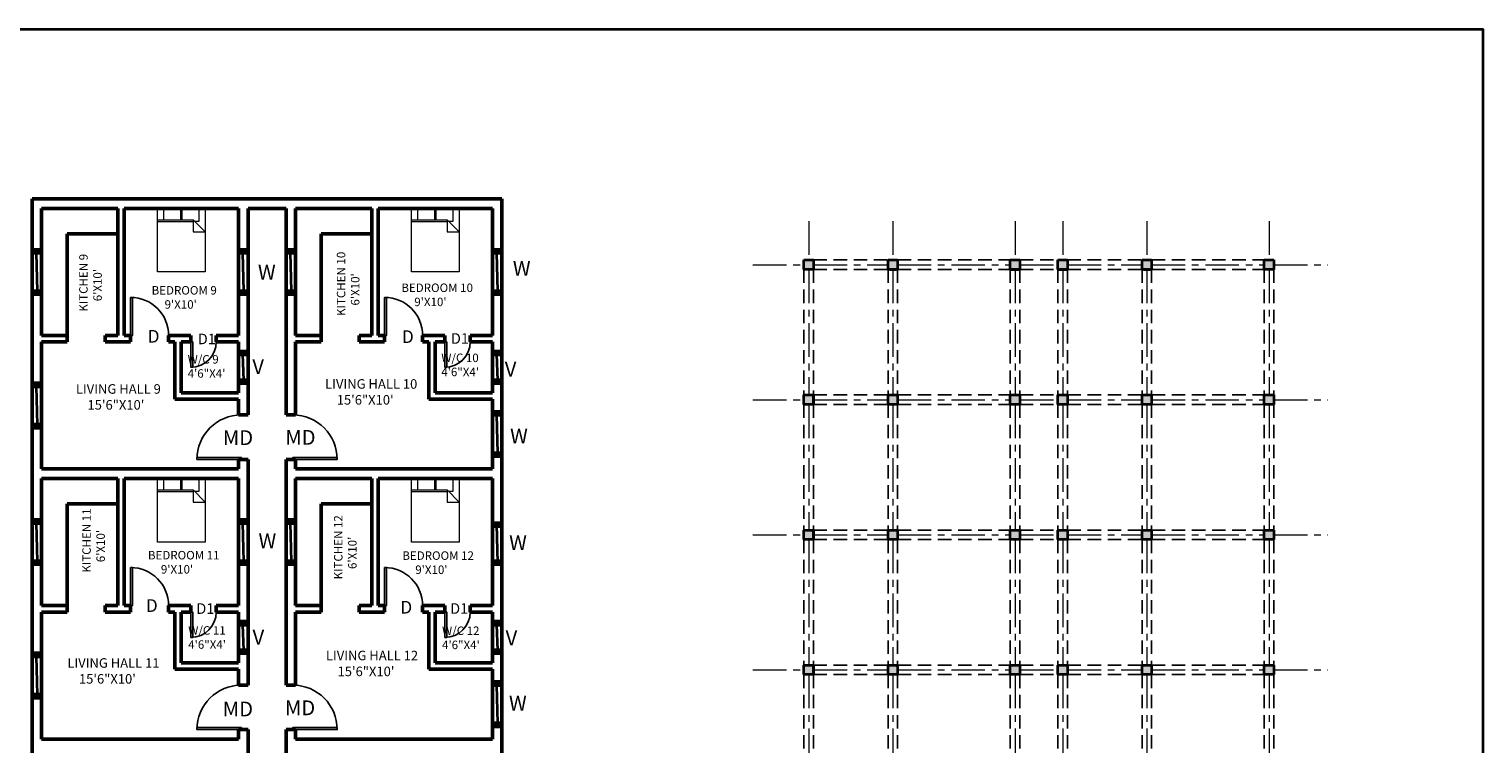
# Model space of a CAD drawing. Units: inches. Extents: x 9239 to 26065, y 6728 to 14611.
# Tile 12 of 12: x 24691 to 26065, y 13937 to 14611. Entities that reach past the tile are written whole.
import ezdxf

# ---------------------------------------------------------------- set-up
doc = ezdxf.new("R2010")
doc.units = ezdxf.units.IN
doc.header["$MEASUREMENT"] = 0
doc.linetypes.add('CENTER', pattern=[50.8, 31.75, -6.35, 6.35, -6.35])
doc.linetypes.add('DASHED', pattern=[19.05, 12.7, -6.35])
for name, color, linetype, lineweight in [('A-ANNO-TEXT', 7, 'Continuous', 18), ('A-ANNO-TTLB', 7, 'Continuous', 35), ('A-AREA-IDEN', 7, 'Continuous', 18), ('A-DOOR', 4, 'Continuous', 25), ('A-FURN', 8, 'Continuous', 18), ('A-GLAZ', 4, 'Continuous', 25), ('A-GRID', 3, 'CENTER', 18), ('A-WALL', 7, 'Continuous', 50), ('S-BEAM', 4, 'DASHED', 25), ('S-COLS', 1, 'Continuous', 35), ('S-PATT', 252, 'Continuous', 13)]:
    doc.layers.add(name, color=color, linetype=linetype, lineweight=lineweight)
doc.styles.get("Standard").update_dxf_attribs({"font": 'arial.ttf'})

# ---------------------------------------------------------------- blocks, each defined once
blk = doc.blocks.new('*U10')
for p, q in [((0, 0), (0, -6)), ((36, 0), (36, -6))]:
    blk.add_line(p, q)
blk.add_lwpolyline([(0, 0), (0, 36), (1.75, 36), (1.75, 0)], close=True)
blk.add_arc((0, 0), 36, 0, 90)
blk = doc.blocks.new('*U34')
for p, q in [((0, 0), (0, 6)), ((24, 0), (24, 6))]:
    blk.add_line(p, q)
blk.add_lwpolyline([(0, 0), (0, -24), (1.75, -24), (1.75, 0)], close=True)
blk.add_arc((0, 0), 24, 270, 0)
blk = doc.blocks.new('*U33')
for p, q in [((-40, 0), (-40, 6)), ((0, 0), (0, 6))]:
    blk.add_line(p, q)
blk.add_lwpolyline([(0, 0), (0, -40), (-1.75, -40), (-1.75, 0)], close=True)
blk.add_arc((0, 0), 40, 180, 270)
blk = doc.blocks.new('*U35')
for p, q in [((0, 0), (0, -6)), ((-40, 0), (-40, -6))]:
    blk.add_line(p, q)
blk.add_lwpolyline([(0, 0), (0, 40), (-1.75, 40), (-1.75, 0)], close=True)
blk.add_arc((0, 0), 40, 90, 180)
blk = doc.blocks.new('Bed - Queen')
for p, q in [((0, -80.00003), (0, 0)), ((0, 0), (59.99999, 0)), ((59.99999, 0), (59.99999, -80.00003)), ((0, -14.4), (44.8, -14.4)), ((44.8, -16.8), (0, -16.8)), ((7.99999, -1.2), (28.79998, -1.2)), ((7.99999, -14.4), (7.99999, -1.2)), ((28.79998, -1.2), (28.79998, -14.4)), ((31.19999, -1.2), (51.99999, -1.2)), ((31.19999, -14.4), (31.19999, -1.2)), ((59.99999, -29.6), (44.8, -14.4)), ((44.8, -14.4), (44.8, -29.6)), ((51.99999, -16.4), (46.79936, -16.4)), ((51.99999, -1.2), (51.99999, -16.4)), ((44.8, -29.6), (59.99999, -29.6)), ((59.99999, -80.00003), (0, -80.00003))]:
    blk.add_line(p, q)
blk = doc.blocks.new('WIN-36')
for p, q in [((0, 1), (36, 1)), ((0, 0.5), (36, 0.5)), ((0, 0), (36, 0))]:
    blk.add_line(p, q)
blk = doc.blocks.new('WIN-24')
for p, q in [((0, 1), (24, 1)), ((0, 0.5), (24, 0.5)), ((0, 0), (24, 0))]:
    blk.add_line(p, q)

msp = doc.modelspace()

# ---------------------------------------------------------------- hatches: boundary and pattern name
at = {"layer": 'S-PATT'}
h = msp.add_hatch(color=256, dxfattribs=at)
h.dxf.hatch_style = 1
h.paths.add_polyline_path([(25432.02, 14384.38), (25432.02, 14393.38), (25423.02, 14393.38), (25423.02, 14384.38)])
h.paths.add_polyline_path([(25511.52, 14384.38), (25511.52, 14393.38), (25502.52, 14393.38), (25502.52, 14384.38)])
h.paths.add_polyline_path([(25627.02, 14384.38), (25627.02, 14393.38), (25618.02, 14393.38), (25618.02, 14384.38)])
h.paths.add_polyline_path([(25672.02, 14393.38), (25663.02, 14393.38), (25663.02, 14384.38), (25672.02, 14384.38)])
h.paths.add_polyline_path([(25742.52, 14384.38), (25751.52, 14384.38), (25751.52, 14393.38), (25742.52, 14393.38)])
h.paths.add_polyline_path([(25858.02, 14384.38), (25867.02, 14384.38), (25867.02, 14393.38), (25858.02, 14393.38)])
h.paths.add_polyline_path([(25423.02, 14256.88), (25432.02, 14256.88), (25432.02, 14265.88), (25423.02, 14265.88)])
h.paths.add_polyline_path([(25502.52, 14256.88), (25511.52, 14256.88), (25511.52, 14265.88), (25502.52, 14265.88)])
h.paths.add_polyline_path([(25618.02, 14256.88), (25627.02, 14256.88), (25627.02, 14265.88), (25618.02, 14265.88)])
h.paths.add_polyline_path([(25672.02, 14265.88), (25663.02, 14265.88), (25663.02, 14256.88), (25672.02, 14256.88)])
h.paths.add_polyline_path([(25751.52, 14256.88), (25751.52, 14265.88), (25742.52, 14265.88), (25742.52, 14256.88)])
h.paths.add_polyline_path([(25858.02, 14256.88), (25867.02, 14256.88), (25867.02, 14265.88), (25858.02, 14265.88)])
h.paths.add_polyline_path([(25423.02, 14129.38), (25432.02, 14129.38), (25432.02, 14138.38), (25423.02, 14138.38)])
h.paths.add_polyline_path([(25511.52, 14129.38), (25511.52, 14138.38), (25502.52, 14138.38), (25502.52, 14129.38)])
h.paths.add_polyline_path([(25618.02, 14129.38), (25627.02, 14129.38), (25627.02, 14138.38), (25618.02, 14138.38)])
h.paths.add_polyline_path([(25672.02, 14138.38), (25663.02, 14138.38), (25663.02, 14129.38), (25672.02, 14129.38)])
h.paths.add_polyline_path([(25742.52, 14129.38), (25751.52, 14129.38), (25751.52, 14138.38), (25742.52, 14138.38)])
h.paths.add_polyline_path([(25867.02, 14129.38), (25867.02, 14138.38), (25858.02, 14138.38), (25858.02, 14129.38)])
h.paths.add_polyline_path([(25432.02, 14010.88), (25423.02, 14010.88), (25423.02, 14001.88), (25432.02, 14001.88)])
h.paths.add_polyline_path([(25502.52, 14010.88), (25502.52, 14001.88), (25511.52, 14001.88), (25511.52, 14010.88)])
h.paths.add_polyline_path([(25618.02, 14001.88), (25627.02, 14001.88), (25627.02, 14010.88), (25618.02, 14010.88)])
h.paths.add_polyline_path([(25672.02, 14001.88), (25672.02, 14010.88), (25663.02, 14010.88), (25663.02, 14001.88)])
h.paths.add_polyline_path([(25751.52, 14010.88), (25742.52, 14010.88), (25742.52, 14001.88), (25751.52, 14001.88)])
h.paths.add_polyline_path([(25867.02, 14010.88), (25858.02, 14010.88), (25858.02, 14001.88), (25867.02, 14001.88)])
h.paths.add_polyline_path([(25432.02, 13874.38), (25432.02, 13883.38), (25423.02, 13883.38), (25423.02, 13874.38)])
h.paths.add_polyline_path([(25502.52, 13874.38), (25511.52, 13874.38), (25511.52, 13883.38), (25502.52, 13883.38)])
h.paths.add_polyline_path([(25627.02, 13883.38), (25618.02, 13883.38), (25618.02, 13874.38), (25627.02, 13874.38)])
h.paths.add_polyline_path([(25672.02, 13874.38), (25672.02, 13883.38), (25663.02, 13883.38), (25663.02, 13874.38)])
h.paths.add_polyline_path([(25751.52, 13883.38), (25742.52, 13883.38), (25742.52, 13874.38), (25751.52, 13874.38)])
h.paths.add_polyline_path([(25858.02, 13874.38), (25867.02, 13874.38), (25867.02, 13883.38), (25858.02, 13883.38)])
h.paths.add_polyline_path([(25432.02, 13746.88), (25432.02, 13755.88), (25423.02, 13755.88), (25423.02, 13746.88)])
h.paths.add_polyline_path([(25502.52, 13747.4), (25511.52, 13747.4), (25511.52, 13756.4), (25502.52, 13756.4)])
h.paths.add_polyline_path([(25627.02, 13746.88), (25627.02, 13755.88), (25618.02, 13755.88), (25618.02, 13746.88)])
h.paths.add_polyline_path([(25672.02, 13746.88), (25672.02, 13755.88), (25663.02, 13755.88), (25663.02, 13746.88)])
h.paths.add_polyline_path([(25742.52, 13746.88), (25751.52, 13746.88), (25751.52, 13755.88), (25742.52, 13755.88)])
h.paths.add_polyline_path([(25867.02, 13746.88), (25867.02, 13755.88), (25858.02, 13755.88), (25858.02, 13746.88)])
h.paths.add_polyline_path([(25423.02, 13619.38), (25432.02, 13619.38), (25432.02, 13628.38), (25423.02, 13628.38)])
h.paths.add_polyline_path([(25511.52, 13619.38), (25511.52, 13628.38), (25502.52, 13628.38), (25502.52, 13619.38)])
h.paths.add_polyline_path([(25627.02, 13619.38), (25627.02, 13628.38), (25618.02, 13628.38), (25618.02, 13619.38)])
h.paths.add_polyline_path([(25672.02, 13619.38), (25672.02, 13628.38), (25663.02, 13628.38), (25663.02, 13619.38)])
h.paths.add_polyline_path([(25751.52, 13628.38), (25742.52, 13628.38), (25742.52, 13619.38), (25751.52, 13619.38)])
h.paths.add_polyline_path([(25858.02, 13619.38), (25867.02, 13619.38), (25867.02, 13628.38), (25858.02, 13628.38)])
h.paths.add_polyline_path([(25423.02, 13491.88), (25432.02, 13491.88), (25432.02, 13500.88), (25423.02, 13500.88)])
h.paths.add_polyline_path([(25511.52, 13500.88), (25502.52, 13500.88), (25502.52, 13491.88), (25511.52, 13491.88)])
h.paths.add_polyline_path([(25627.02, 13491.88), (25627.02, 13500.88), (25618.02, 13500.88), (25618.02, 13491.88)])
h.paths.add_polyline_path([(25663.02, 13491.88), (25672.02, 13491.88), (25672.02, 13500.88), (25663.02, 13500.88)])
h.paths.add_polyline_path([(25742.52, 13491.88), (25751.52, 13491.88), (25751.52, 13500.88), (25742.52, 13500.88)])
h.paths.add_polyline_path([(25432.02, 13373.38), (25423.02, 13373.38), (25423.02, 13364.38), (25432.02, 13364.38)])
h.paths.add_polyline_path([(25502.52, 13373.38), (25502.52, 13364.38), (25511.52, 13364.38), (25511.52, 13373.38)])
h.paths.add_polyline_path([(25618.02, 13373.38), (25618.02, 13364.38), (25627.02, 13364.38), (25627.02, 13373.38)])
h.paths.add_polyline_path([(25663.02, 13373.38), (25663.02, 13364.38), (25672.02, 13364.38), (25672.02, 13373.38)])
h.paths.add_polyline_path([(25742.52, 13373.38), (25742.52, 13364.38), (25751.52, 13364.38), (25751.52, 13373.38)])
h.paths.add_polyline_path([(25858.02, 13373.38), (25858.02, 13364.38), (25867.02, 13364.38), (25867.02, 13373.38)])
h.paths.add_polyline_path([(25432.02, 13298.38), (25423.02, 13298.38), (25423.02, 13289.38), (25432.02, 13289.38)])
h.paths.add_polyline_path([(25511.52, 13298.38), (25502.52, 13298.38), (25502.52, 13289.38), (25511.52, 13289.38)])
h.paths.add_polyline_path([(25618.02, 13298.38), (25618.02, 13289.38), (25627.02, 13289.38), (25627.02, 13298.38)])
h.paths.add_polyline_path([(25663.02, 13298.38), (25663.02, 13289.38), (25672.02, 13289.38), (25672.02, 13298.38)])
h.paths.add_polyline_path([(25742.52, 13298.38), (25742.52, 13289.38), (25751.52, 13289.38), (25751.52, 13298.38)])
h.paths.add_polyline_path([(25858.02, 13298.38), (25858.02, 13289.38), (25867.02, 13289.38), (25867.02, 13298.38)])

# ---------------------------------------------------------------- linework, layer by layer
at = {"layer": 'A-ANNO-TTLB'}
msp.add_lwpolyline([(23324.14, 14611.25), (26064.6, 14611.25), (26064.6, 11591.84), (23324.14, 11591.84)], close=True, dxfattribs=at)
at = {"layer": 'A-GRID'}
for p, q in [((25427.52, 14430.01), (25427.52, 14393.38)), ((25507.02, 14430.01), (25507.02, 14393.38)), ((25622.52, 14430.01), (25622.52, 14393.38)), ((25667.52, 14430.01), (25667.52, 14393.38)), ((25747.02, 14430.01), (25747.02, 14393.38)), ((25862.52, 14430.01), (25862.52, 14393.38)), ((25374.85, 14388.88), (25423.02, 14388.88)), ((25427.52, 14384.38), (25427.52, 14265.88)), ((25432.02, 14388.88), (25502.52, 14388.88)), ((25507.02, 14384.38), (25507.02, 14265.88)), ((25511.52, 14388.88), (25618.02, 14388.88)), ((25622.52, 14384.38), (25622.52, 14265.88)), ((25627.02, 14388.88), (25663.02, 14388.88)), ((25667.52, 14384.38), (25667.52, 14265.88)), ((25672.02, 14388.88), (25742.52, 14388.88)), ((25747.02, 14384.38), (25747.02, 14265.88)), ((25751.52, 14388.88), (25858.02, 14388.88)), ((25862.52, 14384.38), (25862.52, 14265.88)), ((25867.02, 14388.88), (25917.98, 14388.88)), ((25374.85, 14261.38), (25423.02, 14261.38)), ((25432.02, 14261.38), (25502.52, 14261.38)), ((25511.52, 14261.38), (25618.02, 14261.38)), ((25627.02, 14261.38), (25663.02, 14261.38)), ((25672.02, 14261.38), (25742.52, 14261.38)), ((25751.52, 14261.38), (25858.02, 14261.38)), ((25867.02, 14261.38), (25917.98, 14261.38)), ((25427.52, 14256.88), (25427.52, 14138.38)), ((25507.02, 14256.88), (25507.02, 14138.38)), ((25622.52, 14256.88), (25622.52, 14138.38)), ((25667.52, 14256.88), (25667.52, 14138.38)), ((25747.02, 14256.88), (25747.02, 14138.38)), ((25862.52, 14256.88), (25862.52, 14138.38)), ((25374.85, 14133.88), (25423.02, 14133.88)), ((25427.52, 14129.38), (25427.52, 14010.88)), ((25432.02, 14133.88), (25502.52, 14133.88)), ((25507.02, 14129.38), (25507.02, 14010.88)), ((25511.52, 14133.88), (25618.02, 14133.88)), ((25622.52, 14129.38), (25622.52, 14010.88)), ((25627.02, 14133.88), (25663.02, 14133.88)), ((25667.52, 14129.38), (25667.52, 14010.88)), ((25672.02, 14133.88), (25742.52, 14133.88)), ((25747.02, 14129.38), (25747.02, 14010.88)), ((25751.52, 14133.88), (25858.02, 14133.88)), ((25862.52, 14129.38), (25862.52, 14010.88)), ((25867.02, 14133.88), (25917.98, 14133.88)), ((25374.85, 14006.38), (25423.02, 14006.38)), ((25427.52, 14001.88), (25427.52, 13883.38)), ((25432.02, 14006.38), (25502.52, 14006.38)), ((25507.02, 14001.88), (25507.02, 13883.38)), ((25511.52, 14006.38), (25618.02, 14006.38)), ((25622.52, 14001.88), (25622.52, 13883.38)), ((25627.02, 14006.38), (25663.02, 14006.38)), ((25667.52, 14001.88), (25667.52, 13883.38)), ((25672.02, 14006.38), (25742.52, 14006.38)), ((25747.02, 14001.88), (25747.02, 13883.38)), ((25751.52, 14006.38), (25858.02, 14006.38)), ((25862.52, 14001.88), (25862.52, 13883.38)), ((25867.02, 14006.38), (25917.98, 14006.38))]:
    msp.add_line(p, q, dxfattribs=at)
at = {"layer": 'A-WALL'}
for p, q in [((24693.68, 14451.02), (25137.68, 14451.02)), ((24693.68, 13347.02), (24693.68, 14451.02)), ((24702.68, 14442.02), (24774.68, 14442.02)), ((24702.68, 14322.02), (24702.68, 14442.02)), ((24774.68, 14322.02), (24774.68, 14442.02)), ((24780.68, 14322.02), (24780.68, 14442.02)), ((24780.68, 14442.02), (24888.68, 14442.02)), ((24888.68, 14322.02), (24888.68, 14442.02)), ((24897.68, 14247.02), (24897.68, 14442.02)), ((24897.68, 14442.02), (24933.68, 14442.02)), ((24933.68, 14442.02), (24933.68, 14247.02)), ((24942.68, 14442.02), (24942.68, 14322.02)), ((24942.68, 14442.02), (25014.68, 14442.02)), ((25014.68, 14442.02), (25014.68, 14322.02)), ((25020.68, 14442.02), (25020.68, 14322.02)), ((25020.68, 14442.02), (25128.68, 14442.02)), ((25128.68, 14442.02), (25128.68, 14322.02)), ((25137.68, 14451.02), (25137.68, 13347.02)), ((24726.68, 14322.02), (24726.68, 14418.02)), ((24726.68, 14418.02), (24774.68, 14418.02)), ((24966.68, 14418.02), (24966.68, 14322.02)), ((24966.68, 14418.02), (25014.68, 14418.02)), ((24702.68, 14403.02), (24693.68, 14403.02)), ((24702.68, 14400.02), (24693.68, 14400.02)), ((24888.68, 14403.02), (24897.68, 14403.02)), ((24888.68, 14400.02), (24897.68, 14400.02)), ((24942.68, 14403.02), (24933.68, 14403.02)), ((24942.68, 14400.02), (24933.68, 14400.02)), ((25128.68, 14403.02), (25137.68, 14403.02)), ((25128.68, 14400.02), (25137.68, 14400.02)), ((24702.68, 14364.02), (24693.68, 14364.02)), ((24702.68, 14361.02), (24693.68, 14361.02)), ((24888.68, 14364.02), (24897.68, 14364.02)), ((24888.68, 14361.02), (24897.68, 14361.02)), ((24942.68, 14364.02), (24933.68, 14364.02)), ((24942.68, 14361.02), (24933.68, 14361.02)), ((25128.68, 14364.02), (25137.68, 14364.02)), ((25128.68, 14361.02), (25137.68, 14361.02)), ((24702.68, 14322.02), (24726.68, 14322.02)), ((24702.68, 14316.02), (24726.68, 14316.02)), ((24702.68, 14196.02), (24702.68, 14316.02)), ((24726.68, 14316.02), (24726.68, 14322.02)), ((24762.68, 14316.02), (24762.68, 14322.02)), ((24762.68, 14322.02), (24774.68, 14322.02)), ((24762.68, 14316.02), (24786.68, 14316.02)), ((24780.68, 14322.02), (24786.68, 14322.02)), ((24786.68, 14316.02), (24786.68, 14322.02)), ((24822.68, 14316.02), (24822.68, 14322.02)), ((24822.68, 14322.02), (24843.68, 14322.02)), ((24822.68, 14316.02), (24828.68, 14316.02)), ((24828.68, 14262.02), (24828.68, 14316.02)), ((24834.68, 14268.02), (24834.68, 14316.02)), ((24834.68, 14316.02), (24843.68, 14316.02)), ((24843.68, 14316.02), (24843.68, 14322.02)), ((24867.68, 14316.02), (24867.68, 14322.02)), ((24867.68, 14322.02), (24888.68, 14322.02)), ((24867.68, 14316.02), (24888.68, 14316.02)), ((24888.68, 14268.02), (24888.68, 14316.02)), ((24942.68, 14322.02), (24966.68, 14322.02)), ((24942.68, 14316.02), (24966.68, 14316.02)), ((24942.68, 14316.02), (24942.68, 14247.02)), ((24966.68, 14322.02), (24966.68, 14316.02)), ((25002.68, 14322.02), (25002.68, 14316.02)), ((25002.68, 14322.02), (25014.68, 14322.02)), ((25002.68, 14316.02), (25026.68, 14316.02)), ((25020.68, 14322.02), (25026.68, 14322.02)), ((25026.68, 14322.02), (25026.68, 14316.02)), ((25062.68, 14322.02), (25062.68, 14316.02)), ((25062.68, 14322.02), (25083.68, 14322.02)), ((25062.68, 14316.02), (25068.68, 14316.02)), ((25068.68, 14316.02), (25068.68, 14262.02)), ((25074.68, 14316.02), (25074.68, 14268.02)), ((25074.68, 14316.02), (25083.68, 14316.02)), ((25083.68, 14322.02), (25083.68, 14316.02)), ((25107.68, 14322.02), (25107.68, 14316.02)), ((25107.68, 14322.02), (25128.68, 14322.02)), ((25107.68, 14316.02), (25128.68, 14316.02)), ((25128.68, 14316.02), (25128.68, 14268.02)), ((24888.68, 14307.02), (24897.68, 14307.02)), ((24888.68, 14304.02), (24897.68, 14304.02)), ((25128.68, 14307.02), (25137.68, 14307.02)), ((25128.68, 14304.02), (25137.68, 14304.02)), ((24702.68, 14277.02), (24693.68, 14277.02)), ((24702.68, 14274.02), (24693.68, 14274.02)), ((24888.68, 14280.02), (24897.68, 14280.02)), ((24888.68, 14277.02), (24897.68, 14277.02)), ((25128.68, 14280.02), (25137.68, 14280.02)), ((25128.68, 14277.02), (25137.68, 14277.02)), ((24828.68, 14262.02), (24888.68, 14262.02)), ((24834.68, 14268.02), (24888.68, 14268.02)), ((24888.68, 14247.02), (24888.68, 14262.02)), ((25068.68, 14262.02), (25128.68, 14262.02)), ((25074.68, 14268.02), (25128.68, 14268.02)), ((25128.68, 14262.02), (25128.68, 14196.02)), ((24888.68, 14247.02), (24897.68, 14247.02)), ((24933.68, 14247.02), (24942.68, 14247.02)), ((25128.68, 14250.02), (25137.68, 14250.02)), ((25128.68, 14247.02), (25137.68, 14247.02)), ((24702.68, 14238.02), (24693.68, 14238.02)), ((24702.68, 14235.02), (24693.68, 14235.02)), ((24888.68, 14205.02), (24897.68, 14205.02)), ((24888.68, 14196.02), (24888.68, 14205.02)), ((24897.68, 13992.02), (24897.68, 14205.02)), ((24933.68, 14205.02), (24942.68, 14205.02)), ((24933.68, 14205.02), (24933.68, 13992.02)), ((24942.68, 14205.02), (24942.68, 14196.02)), ((25128.68, 14211.02), (25137.68, 14211.02)), ((25128.68, 14208.02), (25137.68, 14208.02)), ((24702.68, 14196.02), (24888.68, 14196.02)), ((24942.68, 14196.02), (25128.68, 14196.02)), ((24702.68, 14187.02), (24774.68, 14187.02)), ((24702.68, 14067.02), (24702.68, 14187.02)), ((24774.68, 14067.02), (24774.68, 14187.02)), ((24780.68, 14067.02), (24780.68, 14187.02)), ((24780.68, 14187.02), (24888.68, 14187.02)), ((24888.68, 14067.02), (24888.68, 14187.02)), ((24942.68, 14187.02), (25014.68, 14187.02)), ((24942.68, 14187.02), (24942.68, 14067.02)), ((25014.68, 14187.02), (25014.68, 14067.02)), ((25020.68, 14187.02), (25020.68, 14067.02)), ((25020.68, 14187.02), (25128.68, 14187.02)), ((25128.68, 14187.02), (25128.68, 14067.02)), ((24726.68, 14067.02), (24726.68, 14163.02)), ((24726.68, 14163.02), (24774.68, 14163.02)), ((24966.68, 14163.02), (24966.68, 14067.02)), ((24966.68, 14163.02), (25014.68, 14163.02)), ((24702.68, 14148.02), (24693.68, 14148.02)), ((24702.68, 14145.02), (24693.68, 14145.02)), ((24888.68, 14148.02), (24897.68, 14148.02)), ((24888.68, 14145.02), (24897.68, 14145.02)), ((24942.68, 14148.02), (24933.68, 14148.02)), ((24942.68, 14145.02), (24933.68, 14145.02)), ((25128.68, 14145.02), (25137.68, 14145.02)), ((25128.68, 14142.02), (25137.68, 14142.02)), ((24702.68, 14109.02), (24693.68, 14109.02)), ((24888.68, 14109.02), (24897.68, 14109.02)), ((24942.68, 14109.02), (24933.68, 14109.02)), ((25128.68, 14109.02), (25137.68, 14109.02)), ((24702.68, 14106.02), (24693.68, 14106.02)), ((24888.68, 14106.02), (24897.68, 14106.02)), ((24942.68, 14106.02), (24933.68, 14106.02)), ((25128.68, 14106.02), (25137.68, 14106.02)), ((24702.68, 14067.02), (24726.68, 14067.02)), ((24702.68, 14061.02), (24726.68, 14061.02)), ((24702.68, 13941.02), (24702.68, 14061.02)), ((24726.68, 14061.02), (24726.68, 14067.02)), ((24762.68, 14061.02), (24762.68, 14067.02)), ((24762.68, 14067.02), (24774.68, 14067.02)), ((24762.68, 14061.02), (24786.68, 14061.02)), ((24780.68, 14067.02), (24786.68, 14067.02)), ((24786.68, 14061.02), (24786.68, 14067.02)), ((24822.68, 14061.02), (24822.68, 14067.02)), ((24822.68, 14067.02), (24843.68, 14067.02)), ((24822.68, 14061.02), (24828.68, 14061.02)), ((24828.68, 14007.02), (24828.68, 14061.02)), ((24834.68, 14013.02), (24834.68, 14061.02)), ((24834.68, 14061.02), (24843.68, 14061.02)), ((24843.68, 14061.02), (24843.68, 14067.02)), ((24867.68, 14061.02), (24867.68, 14067.02)), ((24867.68, 14067.02), (24888.68, 14067.02)), ((24867.68, 14061.02), (24888.68, 14061.02)), ((24888.68, 14013.02), (24888.68, 14061.02)), ((24942.68, 14067.02), (24966.68, 14067.02)), ((24942.68, 14061.02), (24966.68, 14061.02)), ((24942.68, 14061.02), (24942.68, 13992.02)), ((24966.68, 14067.02), (24966.68, 14061.02)), ((25002.68, 14067.02), (25002.68, 14061.02)), ((25002.68, 14067.02), (25014.68, 14067.02)), ((25002.68, 14061.02), (25026.68, 14061.02)), ((25020.68, 14067.02), (25026.68, 14067.02)), ((25026.68, 14067.02), (25026.68, 14061.02)), ((25062.68, 14067.02), (25062.68, 14061.02)), ((25062.68, 14067.02), (25083.68, 14067.02)), ((25062.68, 14061.02), (25068.68, 14061.02)), ((25068.68, 14061.02), (25068.68, 14007.02)), ((25074.68, 14061.02), (25074.68, 14013.02)), ((25074.68, 14061.02), (25083.68, 14061.02)), ((25083.68, 14067.02), (25083.68, 14061.02)), ((25107.68, 14067.02), (25107.68, 14061.02)), ((25107.68, 14067.02), (25128.68, 14067.02)), ((25107.68, 14061.02), (25128.68, 14061.02)), ((25128.68, 14061.02), (25128.68, 14013.02)), ((24888.68, 14052.02), (24897.68, 14052.02)), ((24888.68, 14049.02), (24897.68, 14049.02)), ((25128.68, 14052.02), (25137.68, 14052.02)), ((25128.68, 14049.02), (25137.68, 14049.02)), ((24702.68, 14022.02), (24693.68, 14022.02)), ((24702.68, 14019.02), (24693.68, 14019.02)), ((24834.68, 14013.02), (24888.68, 14013.02)), ((24888.68, 14025.02), (24897.68, 14025.02)), ((24888.68, 14022.02), (24897.68, 14022.02)), ((25074.68, 14013.02), (25128.68, 14013.02)), ((25128.68, 14025.02), (25137.68, 14025.02)), ((25128.68, 14022.02), (25137.68, 14022.02)), ((24828.68, 14007.02), (24888.68, 14007.02)), ((24888.68, 13992.02), (24888.68, 14007.02)), ((25068.68, 14007.02), (25128.68, 14007.02)), ((25128.68, 14007.02), (25128.68, 13941.02)), ((24888.68, 13992.02), (24897.68, 13992.02)), ((24933.68, 13992.02), (24942.68, 13992.02)), ((25128.68, 13995.02), (25137.68, 13995.02)), ((25128.68, 13992.02), (25137.68, 13992.02)), ((24702.68, 13983.02), (24693.68, 13983.02)), ((24702.68, 13980.02), (24693.68, 13980.02)), ((24888.68, 13950.02), (24897.68, 13950.02)), ((24888.68, 13941.02), (24888.68, 13950.02)), ((24897.68, 13737.02), (24897.68, 13950.02)), ((24933.68, 13950.02), (24942.68, 13950.02)), ((24933.68, 13950.02), (24933.68, 13737.02)), ((24942.68, 13950.02), (24942.68, 13941.02)), ((25128.68, 13956.02), (25137.68, 13956.02)), ((25128.68, 13953.02), (25137.68, 13953.02)), ((24702.68, 13941.02), (24888.68, 13941.02)), ((24942.68, 13941.02), (25128.68, 13941.02))]:
    msp.add_line(p, q, dxfattribs=at)
at = {"layer": 'S-BEAM'}
for p, q in [((25423.02, 14384.38), (25423.02, 14265.88)), ((25432.02, 14393.38), (25502.52, 14393.38)), ((25432.02, 14384.38), (25502.52, 14384.38)), ((25432.02, 14384.38), (25432.02, 14265.88)), ((25502.52, 14384.38), (25502.52, 14265.88)), ((25511.52, 14393.38), (25618.02, 14393.38)), ((25511.52, 14384.38), (25618.02, 14384.38)), ((25511.52, 14384.38), (25511.52, 14265.88)), ((25618.02, 14384.38), (25618.02, 14265.88)), ((25627.02, 14393.38), (25663.02, 14393.38)), ((25627.02, 14384.38), (25663.02, 14384.38)), ((25627.02, 14384.38), (25627.02, 14265.88)), ((25663.02, 14384.38), (25663.02, 14265.88)), ((25672.02, 14393.38), (25742.52, 14393.38)), ((25672.02, 14384.38), (25742.52, 14384.38)), ((25672.02, 14384.38), (25672.02, 14265.88)), ((25742.52, 14384.38), (25742.52, 14265.88)), ((25751.52, 14393.38), (25858.02, 14393.38)), ((25751.52, 14384.38), (25858.02, 14384.38)), ((25751.52, 14384.38), (25751.52, 14265.88)), ((25858.02, 14384.38), (25858.02, 14265.88)), ((25867.02, 14384.38), (25867.02, 14265.88)), ((25432.02, 14265.88), (25502.52, 14265.88)), ((25511.52, 14265.88), (25618.02, 14265.88)), ((25627.02, 14265.88), (25663.02, 14265.88)), ((25672.02, 14265.88), (25742.52, 14265.88)), ((25751.52, 14265.88), (25858.02, 14265.88)), ((25423.02, 14256.88), (25423.02, 14138.38)), ((25432.02, 14256.88), (25502.52, 14256.88)), ((25432.02, 14256.88), (25432.02, 14138.38)), ((25502.52, 14256.88), (25502.52, 14138.38)), ((25511.52, 14256.88), (25618.02, 14256.88)), ((25511.52, 14256.88), (25511.52, 14138.38)), ((25618.02, 14256.88), (25618.02, 14138.38)), ((25627.02, 14256.88), (25663.02, 14256.88)), ((25627.02, 14256.88), (25627.02, 14138.38)), ((25663.02, 14256.88), (25663.02, 14138.38)), ((25672.02, 14256.88), (25742.52, 14256.88)), ((25672.02, 14256.88), (25672.02, 14138.38)), ((25742.52, 14256.88), (25742.52, 14138.38)), ((25751.52, 14256.88), (25858.02, 14256.88)), ((25751.52, 14256.88), (25751.52, 14138.38)), ((25858.02, 14256.88), (25858.02, 14138.38)), ((25867.02, 14256.88), (25867.02, 14138.38)), ((25432.02, 14138.38), (25502.52, 14138.38)), ((25511.52, 14138.38), (25618.02, 14138.38)), ((25627.02, 14138.38), (25663.02, 14138.38)), ((25672.02, 14138.38), (25742.52, 14138.38)), ((25751.52, 14138.38), (25858.02, 14138.38)), ((25423.02, 14129.38), (25423.02, 14010.88)), ((25432.02, 14129.38), (25502.52, 14129.38)), ((25432.02, 14129.38), (25432.02, 14010.88)), ((25502.52, 14129.38), (25502.52, 14010.88)), ((25511.52, 14129.38), (25618.02, 14129.38)), ((25511.52, 14129.38), (25511.52, 14010.88)), ((25618.02, 14129.38), (25618.02, 14010.88)), ((25627.02, 14129.38), (25663.02, 14129.38)), ((25627.02, 14129.38), (25627.02, 14010.88)), ((25663.02, 14129.38), (25663.02, 14010.88)), ((25672.02, 14129.38), (25742.52, 14129.38)), ((25672.02, 14129.38), (25672.02, 14010.88)), ((25742.52, 14129.38), (25742.52, 14010.88)), ((25751.52, 14129.38), (25858.02, 14129.38)), ((25751.52, 14129.38), (25751.52, 14010.88)), ((25858.02, 14129.38), (25858.02, 14010.88)), ((25867.02, 14129.38), (25867.02, 14010.88)), ((25423.02, 14001.88), (25423.02, 13883.38)), ((25432.02, 14010.88), (25502.52, 14010.88)), ((25432.02, 14001.88), (25502.52, 14001.88)), ((25432.02, 14001.88), (25432.02, 13883.38)), ((25502.52, 14001.88), (25502.52, 13883.38)), ((25511.52, 14010.88), (25618.02, 14010.88)), ((25511.52, 14001.88), (25618.02, 14001.88)), ((25511.52, 14001.88), (25511.52, 13883.38)), ((25618.02, 14001.88), (25618.02, 13883.38)), ((25627.02, 14010.88), (25663.02, 14010.88)), ((25627.02, 14001.88), (25663.02, 14001.88)), ((25627.02, 14001.88), (25627.02, 13883.38)), ((25663.02, 14001.88), (25663.02, 13883.38)), ((25672.02, 14010.88), (25742.52, 14010.88)), ((25672.02, 14001.88), (25742.52, 14001.88)), ((25672.02, 14001.88), (25672.02, 13883.38)), ((25742.52, 14001.88), (25742.52, 13883.38)), ((25751.52, 14010.88), (25858.02, 14010.88)), ((25751.52, 14001.88), (25858.02, 14001.88)), ((25751.52, 14001.88), (25751.52, 13883.38)), ((25858.02, 14001.88), (25858.02, 13883.38)), ((25867.02, 14001.88), (25867.02, 13883.38))]:
    msp.add_line(p, q, dxfattribs=at)
at = {"layer": 'S-COLS'}
for p, q in [((25423.02, 14393.38), (25432.02, 14393.38)), ((25423.02, 14384.38), (25423.02, 14393.38)), ((25432.02, 14384.38), (25423.02, 14384.38)), ((25432.02, 14393.38), (25432.02, 14384.38)), ((25502.52, 14393.38), (25511.52, 14393.38)), ((25502.52, 14384.38), (25502.52, 14393.38)), ((25511.52, 14384.38), (25502.52, 14384.38)), ((25504.02, 14384.38), (25510.02, 14384.38)), ((25511.52, 14393.38), (25511.52, 14384.38)), ((25618.02, 14393.38), (25627.02, 14393.38)), ((25618.02, 14384.38), (25618.02, 14393.38)), ((25618.02, 14384.38), (25627.02, 14384.38)), ((25627.02, 14384.38), (25618.02, 14384.38)), ((25627.02, 14393.38), (25627.02, 14384.38)), ((25663.02, 14393.38), (25672.02, 14393.38)), ((25663.02, 14384.38), (25663.02, 14393.38)), ((25663.02, 14384.38), (25672.02, 14384.38)), ((25672.02, 14384.38), (25663.02, 14384.38)), ((25672.02, 14393.38), (25672.02, 14384.38)), ((25742.52, 14393.38), (25751.52, 14393.38)), ((25742.52, 14384.38), (25742.52, 14393.38)), ((25751.52, 14384.38), (25742.52, 14384.38)), ((25744.02, 14384.38), (25750.02, 14384.38)), ((25751.52, 14393.38), (25751.52, 14384.38)), ((25858.02, 14393.38), (25867.02, 14393.38)), ((25858.02, 14384.38), (25858.02, 14393.38)), ((25867.02, 14384.38), (25858.02, 14384.38)), ((25867.02, 14393.38), (25867.02, 14384.38)), ((25423.02, 14265.88), (25432.02, 14265.88)), ((25423.02, 14256.88), (25423.02, 14265.88)), ((25432.02, 14265.88), (25432.02, 14256.88)), ((25432.02, 14258.38), (25432.02, 14264.38)), ((25502.52, 14265.88), (25511.52, 14265.88)), ((25502.52, 14256.88), (25502.52, 14265.88)), ((25511.52, 14265.88), (25511.52, 14256.88)), ((25618.02, 14265.88), (25627.02, 14265.88)), ((25618.02, 14256.88), (25618.02, 14265.88)), ((25627.02, 14265.88), (25627.02, 14256.88)), ((25663.02, 14265.88), (25672.02, 14265.88)), ((25663.02, 14256.88), (25663.02, 14265.88)), ((25672.02, 14265.88), (25672.02, 14256.88)), ((25742.52, 14265.88), (25751.52, 14265.88)), ((25742.52, 14256.88), (25742.52, 14265.88)), ((25751.52, 14265.88), (25751.52, 14256.88)), ((25858.02, 14265.88), (25867.02, 14265.88)), ((25858.02, 14256.88), (25858.02, 14265.88)), ((25867.02, 14265.88), (25867.02, 14256.88)), ((25432.02, 14256.88), (25423.02, 14256.88)), ((25511.52, 14256.88), (25502.52, 14256.88)), ((25627.02, 14256.88), (25618.02, 14256.88)), ((25672.02, 14256.88), (25663.02, 14256.88)), ((25751.52, 14256.88), (25742.52, 14256.88)), ((25867.02, 14256.88), (25858.02, 14256.88)), ((25423.02, 14138.38), (25432.02, 14138.38)), ((25423.02, 14129.38), (25423.02, 14138.38)), ((25432.02, 14129.38), (25432.02, 14138.38)), ((25432.02, 14138.38), (25432.02, 14129.38)), ((25502.52, 14138.38), (25511.52, 14138.38)), ((25502.52, 14129.38), (25502.52, 14138.38)), ((25511.52, 14138.38), (25511.52, 14129.38)), ((25618.02, 14138.38), (25627.02, 14138.38)), ((25618.02, 14129.38), (25618.02, 14138.38)), ((25627.02, 14138.38), (25627.02, 14129.38)), ((25663.02, 14138.38), (25672.02, 14138.38)), ((25663.02, 14129.38), (25663.02, 14138.38)), ((25672.02, 14138.38), (25672.02, 14129.38)), ((25742.52, 14138.38), (25751.52, 14138.38)), ((25742.52, 14129.38), (25742.52, 14138.38)), ((25751.52, 14138.38), (25751.52, 14129.38)), ((25858.02, 14138.38), (25867.02, 14138.38)), ((25858.02, 14129.38), (25858.02, 14138.38)), ((25867.02, 14138.38), (25867.02, 14129.38)), ((25432.02, 14129.38), (25423.02, 14129.38)), ((25511.52, 14129.38), (25502.52, 14129.38)), ((25627.02, 14129.38), (25618.02, 14129.38)), ((25672.02, 14129.38), (25663.02, 14129.38)), ((25751.52, 14129.38), (25742.52, 14129.38)), ((25867.02, 14129.38), (25858.02, 14129.38)), ((25423.02, 14010.88), (25432.02, 14010.88)), ((25423.02, 14001.88), (25423.02, 14010.88)), ((25432.02, 14001.88), (25423.02, 14001.88)), ((25432.02, 14010.88), (25432.02, 14001.88)), ((25432.02, 14003.38), (25432.02, 14009.38)), ((25502.52, 14010.88), (25511.52, 14010.88)), ((25502.52, 14001.88), (25502.52, 14010.88)), ((25511.52, 14001.88), (25502.52, 14001.88)), ((25511.52, 14010.88), (25511.52, 14001.88)), ((25618.02, 14010.88), (25627.02, 14010.88)), ((25618.02, 14001.88), (25618.02, 14010.88)), ((25627.02, 14001.88), (25618.02, 14001.88)), ((25627.02, 14010.88), (25627.02, 14001.88)), ((25663.02, 14010.88), (25672.02, 14010.88)), ((25663.02, 14001.88), (25663.02, 14010.88)), ((25672.02, 14001.88), (25663.02, 14001.88)), ((25672.02, 14010.88), (25672.02, 14001.88)), ((25742.52, 14010.88), (25751.52, 14010.88)), ((25742.52, 14001.88), (25742.52, 14010.88)), ((25751.52, 14001.88), (25742.52, 14001.88)), ((25751.52, 14010.88), (25751.52, 14001.88)), ((25858.02, 14010.88), (25867.02, 14010.88)), ((25858.02, 14001.88), (25858.02, 14010.88)), ((25867.02, 14001.88), (25858.02, 14001.88)), ((25867.02, 14010.88), (25867.02, 14001.88))]:
    msp.add_line(p, q, dxfattribs=at)

# ---------------------------------------------------------------- block references
at = {"layer": 'A-DOOR'}
for name, p in [('*U10', (24786.68, 14322.02)), ('*U10', (25026.68, 14322.02)), ('*U34', (24843.68, 14316.02)), ('*U34', (25083.68, 14316.02)), ('*U10', (24786.68, 14067.02)), ('*U10', (25026.68, 14067.02)), ('*U34', (24843.68, 14061.02)), ('*U34', (25083.68, 14061.02))]:
    msp.add_blockref(name, p, dxfattribs=at)
at = {"layer": 'A-DOOR', "xscale": 1.05, "yscale": 1.05, "zscale": 1.05, "rotation": 270}
for name, p in [('*U33', (24891.38, 14205.02)), ('*U35', (24939.98, 14205.02)), ('*U33', (24891.38, 13950.02)), ('*U35', (24939.98, 13950.02))]:
    msp.add_blockref(name, p, dxfattribs=at)
at = {"layer": 'A-FURN', "xscale": 0.75, "yscale": 0.75, "zscale": 0.75}
for p in [(24812.18, 14442.02), (25052.18, 14442.02), (24812.18, 14187.02), (25052.18, 14187.02)]:
    msp.add_blockref('Bed - Queen', p, dxfattribs=at)
at = {"layer": 'A-GLAZ'}
for name, p, rotation in [('WIN-36', (24697.18, 14400), 271.5911402711772), ('WIN-36', (24892.18, 14400), 271.5911402712003), ('WIN-36', (24937.18, 14400), 271.5911402712003), ('WIN-36', (25132.18, 14400), 271.5911402712003), ('WIN-24', (24892.18, 14303.99), 272.3859440303975), ('WIN-24', (25132.18, 14303.99), 272.3859440303975), ('WIN-36', (24697.18, 14274), 271.5911402711772), ('WIN-36', (25132.18, 14247), 271.5911402712003), ('WIN-36', (24697.18, 14145), 271.5911402711772), ('WIN-36', (24892.18, 14145), 271.5911402712003), ('WIN-36', (24937.18, 14145), 271.5911402712003), ('WIN-36', (25132.18, 14143.5), 271.5911402712003), ('WIN-24', (24892.18, 14048.99), 272.3859440303975), ('WIN-24', (25132.18, 14048.99), 272.3859440303975), ('WIN-36', (24697.18, 14019), 271.5911402712003), ('WIN-36', (25132.18, 13992), 271.5911402712003)]:
    msp.add_blockref(name, p, dxfattribs=dict(at, rotation=rotation))

# ---------------------------------------------------------------- texts
at = {"layer": 'A-ANNO-TEXT', "attachment_point": 1}
for s, width, insert, char_height in [('W', 545.3335, (24907.07, 14388.8), 14), ('W', 545.3335, (25147.94, 14392.44), 14), ('D', 545.3335, (24802.82, 14327.28), 12), ('D1', 545.3335, (24850.27, 14323.78), 10), ('D', 545.3335, (25043.09, 14326.92), 12), ('D1', 545.3335, (25089.45, 14324.19), 10), ('W/C 9\\P4\'6"X4\'', 1026.6179, (24840.66, 14303.54), 8), ('W/C 10\\P4\'6"X4\'', 1026.6179, (25080.33, 14304.96), 8), ('V', 545.3335, (24901.79, 14299.66), 14), ('V', 545.3335, (25140.3, 14297.3), 14), ('MD', 545.3335, (24873.89, 14232.6), 14), ('MD', 545.3335, (24932.91, 14232.84), 14), ('W', 545.3335, (25145.33, 14234.15), 14), ('W', 545.3335, (24907.59, 14135.21), 14), ('W', 545.3335, (25144.41, 14133.53), 14), ('D', 545.3335, (24801.13, 14073.11), 12), ('D1', 545.3335, (24848.88, 14069.24), 10), ('D', 545.3335, (25041.59, 14071.53), 12), ('D1', 545.3335, (25088.76, 14069.3), 10), ('W/C 11\\P4\'6"X4\'', 1026.6179, (24841.19, 14047.64), 8), ('V', 545.3335, (24901.99, 14044.29), 14), ('W/C 12\\P4\'6"X4\'', 1026.6179, (25081.05, 14047.33), 8), ('V', 545.3335, (25141.1, 14043.61), 14), ('MD', 545.3335, (24873.83, 13976.45), 14), ('MD', 545.3335, (24932.56, 13977.57), 14), ('W', 545.3335, (25144.27, 13981.96), 14)]:
    msp.add_mtext_dynamic_manual_height_columns(s, width=width, gutter_width=1, heights=[0], dxfattribs=dict(at, insert=insert, char_height=char_height))
at = {"layer": 'A-AREA-IDEN', "char_height": 8, "attachment_point": 1, "rotation": 90}
for s, insert in [("KITCHEN 9\\P    6'X10'", (24738.19, 14344.56)), ("KITCHEN 10\\P    6'X10'", (24981.62, 14340.52)), ("KITCHEN 11\\P    6'X10'", (24741.11, 14098.24)), ("KITCHEN 12\\P    6'X10'", (24978.95, 14091.82))]:
    msp.add_mtext_dynamic_manual_height_columns(s, width=757.9977, gutter_width=1, heights=[0], dxfattribs=dict(at, insert=insert))
at = {"layer": 'A-AREA-IDEN', "attachment_point": 1}
for s, width, insert, char_height in [("BEDROOM 10\\P     9'X10'", 562.7126, (25042.6, 14371.09), 8), ("BEDROOM 9\\P     9'X10'", 562.7126, (24806.62, 14368.67), 8), ('LIVING HALL 9\\P    15\'6"X10\'', 436.6568, (24735.03, 14276.06), 9), ('LIVING HALL 10\\P    15\'6"X10\'', 436.6568, (24970.53, 14280.81), 9), ("BEDROOM 11\\P     9'X10'", 562.7126, (24803.14, 14118.65), 8), ("BEDROOM 12\\P     9'X10'", 562.7126, (25043.52, 14118.26), 8), ('LIVING HALL 11\\P    15\'6"X10\'', 436.6568, (24726.96, 14017.4), 9), ('LIVING HALL 12\\P    15\'6"X10\'', 436.6568, (24971.31, 14024.44), 9)]:
    msp.add_mtext_dynamic_manual_height_columns(s, width=width, gutter_width=1, heights=[0], dxfattribs=dict(at, insert=insert, char_height=char_height))

doc.saveas('drawing.dxf')
